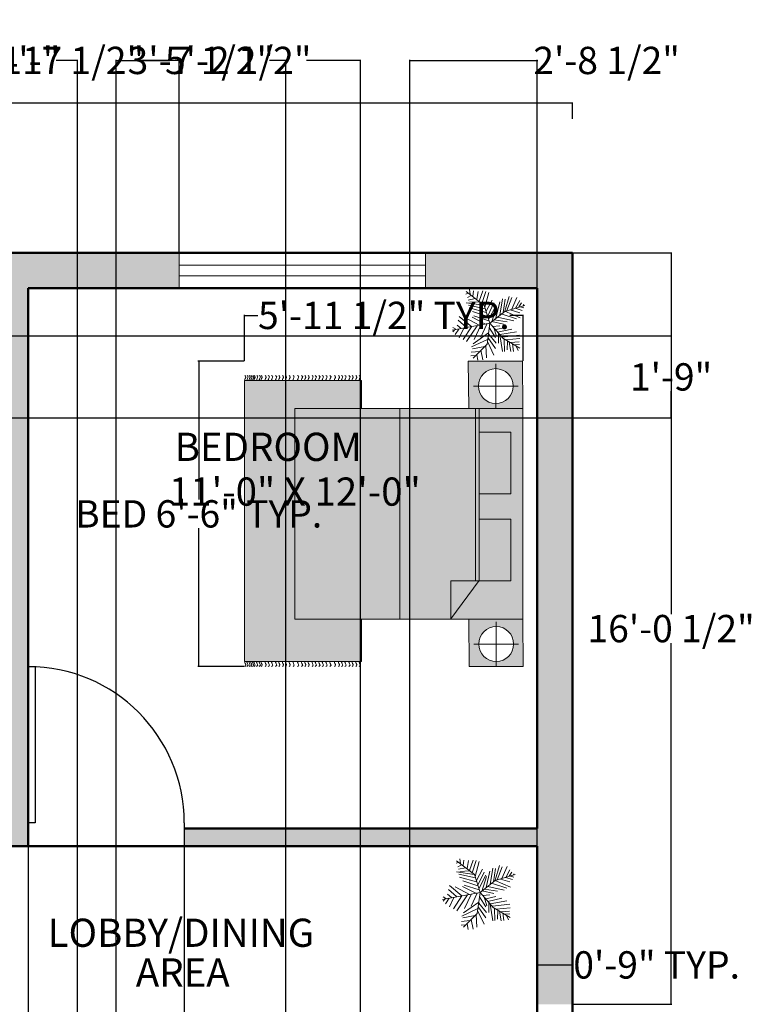
# Model space of a CAD drawing. Units: inches. Extents: x 2974 to 3443, y 2405 to 2963.
# Tile 13 of 13: x 3243 to 3430, y 2711 to 2963. Entities that reach past the tile are written whole.
import ezdxf

# ---------------------------------------------------------------- set-up
doc = ezdxf.new("R2010")
doc.units = ezdxf.units.IN
doc.header["$MEASUREMENT"] = 0
doc.layers.get('0').update_dxf_attribs({"color": 251})
for name, color, linetype, lineweight in [('A-ANNO-DIMS', 2, 'Continuous', 18), ('A-AREA-IDEN', 250, 'Continuous', 25), ('A-DOOR', 32, 'Continuous', 25), ('A-WALL-PATT', 252, 'Continuous', 13), ('furniture', 32, 'Continuous', 18), ('greenary', 106, 'Continuous', 13), ('walls', 250, 'Continuous', 50), ('windows', 159, 'Continuous', 20)]:
    doc.layers.add(name, color=color, linetype=linetype, lineweight=lineweight)
doc.layers.add('A-FURN-PATT', color=254, linetype='Continuous', lineweight=13, true_color=0xfeeab9)
doc.styles.get("Standard").update_dxf_attribs({"font": 'arial.ttf'})
doc.dimstyles.get("Standard").update_dxf_attribs({"dimtxt": 7, "dimasz": 0.18, "dimexe": 0.18, "dimexo": 0.0625, "dimgap": 0.09, "dimtad": 0, "dimtih": 1, "dimtoh": 1, "dimzin": 0, "dimdsep": 46, "dimlunit": 3, "dimtxsty": 'Standard', "dimcen": 0.09, "dimadec": 0, "dimazin": 0, "dimtfac": 1, "dimtofl": 0, "dimtmove": 0, "dimatfit": 3, "dimfxl": 1, "dimtolj": 1, "dimtzin": 0, "dimarcsym": 0})

# ---------------------------------------------------------------- blocks, each defined once
blk = doc.blocks.new('*U2')
for p, q in [((0, 0), (0, -6)), ((40, 0), (40, -6))]:
    blk.add_line(p, q)
blk.add_lwpolyline([(0, 0), (0, 40), (1.75, 40), (1.75, 0)], close=True)
blk.add_arc((0, 0), 40, 0, 90)
blk = doc.blocks.new('CARPET')
at = {"layer": 'furniture'}
for p, q in [((-51.53, -98.11), (-51.53, -55.12)), ((-51.53, -55.12), (-41.27, -55.12)), ((36, -55.12), (51.55, -55.12)), ((51.55, -55.12), (51.55, -98.11)), ((51.55, -98.11), (-51.53, -98.11))]:
    blk.add_line(p, q, dxfattribs=at)
for points, knots in [([(-53.37, -55.99), (-53.22, -55.8), (-52.9, -55.41), (-52.34, -55.8), (-51.89, -56.08), (-51.65, -55.91), (-51.53, -55.83)], [0, 0, 0, 0, 0.653278, 1.290138, 1.740457, 2.114451, 2.114451, 2.114451, 2.114451]), ([(-53.37, -57.26), (-53.22, -57.07), (-52.9, -56.67), (-52.34, -57.07), (-51.89, -57.35), (-51.65, -57.17), (-51.53, -57.1)], [0, 0, 0, 0, 0.653278, 1.290138, 1.740457, 2.114451, 2.114451, 2.114451, 2.114451]), ([(53.37, -55.99), (53.22, -55.8), (52.9, -55.41), (52.34, -55.8), (51.89, -56.08), (51.65, -55.91), (51.53, -55.83)], [0, 0, 0, 0, 0.653278, 1.290138, 1.740457, 2.114451, 2.114451, 2.114451, 2.114451]), ([(53.37, -57.26), (53.22, -57.07), (52.9, -56.67), (52.34, -57.07), (51.89, -57.35), (51.65, -57.17), (51.53, -57.1)], [0, 0, 0, 0, 0.653278, 1.290138, 1.740457, 2.114451, 2.114451, 2.114451, 2.114451]), ([(-53.37, -58.59), (-53.22, -58.4), (-52.9, -58.01), (-52.34, -58.4), (-51.89, -58.68), (-51.65, -58.5), (-51.53, -58.43)], [0, 0, 0, 0, 0.653278, 1.290138, 1.740457, 2.114451, 2.114451, 2.114451, 2.114451]), ([(-53.37, -59.78), (-53.22, -59.58), (-52.9, -59.19), (-52.34, -59.58), (-51.89, -59.86), (-51.65, -59.69), (-51.53, -59.61)], [0, 0, 0, 0, 0.653278, 1.290138, 1.740457, 2.114451, 2.114451, 2.114451, 2.114451]), ([(-53.37, -61.22), (-53.22, -61.02), (-52.9, -60.63), (-52.34, -61.02), (-51.89, -61.3), (-51.65, -61.13), (-51.53, -61.05)], [0, 0, 0, 0, 0.653278, 1.290138, 1.740457, 2.114451, 2.114451, 2.114451, 2.114451]), ([(53.37, -58.59), (53.22, -58.4), (52.9, -58.01), (52.34, -58.4), (51.89, -58.68), (51.65, -58.5), (51.53, -58.43)], [0, 0, 0, 0, 0.653278, 1.290138, 1.740457, 2.114451, 2.114451, 2.114451, 2.114451]), ([(53.37, -59.78), (53.22, -59.58), (52.9, -59.19), (52.34, -59.58), (51.89, -59.86), (51.65, -59.69), (51.53, -59.61)], [0, 0, 0, 0, 0.653278, 1.290138, 1.740457, 2.114451, 2.114451, 2.114451, 2.114451]), ([(53.37, -61.22), (53.22, -61.02), (52.9, -60.63), (52.34, -61.02), (51.89, -61.3), (51.65, -61.13), (51.53, -61.05)], [0, 0, 0, 0, 0.653278, 1.290138, 1.740457, 2.114451, 2.114451, 2.114451, 2.114451]), ([(-53.37, -62.44), (-53.22, -62.25), (-52.9, -61.86), (-52.34, -62.25), (-51.89, -62.53), (-51.65, -62.36), (-51.53, -62.28)], [0, 0, 0, 0, 0.653278, 1.290138, 1.740457, 2.114451, 2.114451, 2.114451, 2.114451]), ([(-53.37, -63.63), (-53.22, -63.43), (-52.9, -63.04), (-52.34, -63.43), (-51.89, -63.72), (-51.65, -63.54), (-51.53, -63.46)], [0, 0, 0, 0, 0.653278, 1.290138, 1.740457, 2.114451, 2.114451, 2.114451, 2.114451]), ([(-53.37, -65.07), (-53.22, -64.87), (-52.9, -64.48), (-52.34, -64.87), (-51.89, -65.15), (-51.65, -64.98), (-51.53, -64.9)], [0, 0, 0, 0, 0.653278, 1.290138, 1.740457, 2.114451, 2.114451, 2.114451, 2.114451]), ([(53.37, -62.44), (53.22, -62.25), (52.9, -61.86), (52.34, -62.25), (51.89, -62.53), (51.65, -62.36), (51.53, -62.28)], [0, 0, 0, 0, 0.653278, 1.290138, 1.740457, 2.114451, 2.114451, 2.114451, 2.114451]), ([(53.37, -63.63), (53.22, -63.43), (52.9, -63.04), (52.34, -63.43), (51.89, -63.72), (51.65, -63.54), (51.53, -63.46)], [0, 0, 0, 0, 0.653278, 1.290138, 1.740457, 2.114451, 2.114451, 2.114451, 2.114451]), ([(53.37, -65.07), (53.22, -64.87), (52.9, -64.48), (52.34, -64.87), (51.89, -65.15), (51.65, -64.98), (51.53, -64.9)], [0, 0, 0, 0, 0.653278, 1.290138, 1.740457, 2.114451, 2.114451, 2.114451, 2.114451]), ([(-53.37, -66.76), (-53.22, -66.56), (-52.9, -66.17), (-52.34, -66.56), (-51.89, -66.84), (-51.65, -66.67), (-51.53, -66.59)], [0, 0, 0, 0, 0.653278, 1.290138, 1.740457, 2.114451, 2.114451, 2.114451, 2.114451]), ([(-53.37, -68.2), (-53.22, -68), (-52.9, -67.61), (-52.34, -68), (-51.89, -68.28), (-51.65, -68.11), (-51.53, -68.03)], [0, 0, 0, 0, 0.653278, 1.290138, 1.740457, 2.114451, 2.114451, 2.114451, 2.114451]), ([(53.37, -66.76), (53.22, -66.56), (52.9, -66.17), (52.34, -66.56), (51.89, -66.84), (51.65, -66.67), (51.53, -66.59)], [0, 0, 0, 0, 0.653278, 1.290138, 1.740457, 2.114451, 2.114451, 2.114451, 2.114451]), ([(53.37, -68.2), (53.22, -68), (52.9, -67.61), (52.34, -68), (51.89, -68.28), (51.65, -68.11), (51.53, -68.03)], [0, 0, 0, 0, 0.653278, 1.290138, 1.740457, 2.114451, 2.114451, 2.114451, 2.114451]), ([(-53.37, -69.53), (-53.22, -69.33), (-52.9, -68.94), (-52.34, -69.33), (-51.89, -69.61), (-51.65, -69.44), (-51.53, -69.36)], [0, 0, 0, 0, 0.653278, 1.290138, 1.740457, 2.114451, 2.114451, 2.114451, 2.114451]), ([(-53.37, -70.79), (-53.22, -70.6), (-52.9, -70.21), (-52.34, -70.6), (-51.89, -70.88), (-51.65, -70.7), (-51.53, -70.63)], [0, 0, 0, 0, 0.653278, 1.290138, 1.740457, 2.114451, 2.114451, 2.114451, 2.114451]), ([(-53.37, -72.12), (-53.22, -71.93), (-52.9, -71.54), (-52.34, -71.93), (-51.89, -72.21), (-51.65, -72.04), (-51.53, -71.96)], [0, 0, 0, 0, 0.653278, 1.290138, 1.740457, 2.114451, 2.114451, 2.114451, 2.114451]), ([(53.37, -69.53), (53.22, -69.33), (52.9, -68.94), (52.34, -69.33), (51.89, -69.61), (51.65, -69.44), (51.53, -69.36)], [0, 0, 0, 0, 0.653278, 1.290138, 1.740457, 2.114451, 2.114451, 2.114451, 2.114451]), ([(53.37, -70.79), (53.22, -70.6), (52.9, -70.21), (52.34, -70.6), (51.89, -70.88), (51.65, -70.7), (51.53, -70.63)], [0, 0, 0, 0, 0.653278, 1.290138, 1.740457, 2.114451, 2.114451, 2.114451, 2.114451]), ([(53.37, -72.12), (53.22, -71.93), (52.9, -71.54), (52.34, -71.93), (51.89, -72.21), (51.65, -72.04), (51.53, -71.96)], [0, 0, 0, 0, 0.653278, 1.290138, 1.740457, 2.114451, 2.114451, 2.114451, 2.114451]), ([(-53.37, -73.31), (-53.22, -73.11), (-52.9, -72.72), (-52.34, -73.11), (-51.89, -73.4), (-51.65, -73.22), (-51.53, -73.14)], [0, 0, 0, 0, 0.653278, 1.290138, 1.740457, 2.114451, 2.114451, 2.114451, 2.114451]), ([(-53.37, -74.75), (-53.22, -74.55), (-52.9, -74.16), (-52.34, -74.55), (-51.89, -74.83), (-51.65, -74.66), (-51.53, -74.58)], [0, 0, 0, 0, 0.653278, 1.290138, 1.740457, 2.114451, 2.114451, 2.114451, 2.114451]), ([(-53.37, -75.98), (-53.22, -75.78), (-52.9, -75.39), (-52.34, -75.78), (-51.89, -76.06), (-51.65, -75.89), (-51.53, -75.81)], [0, 0, 0, 0, 0.653278, 1.290138, 1.740457, 2.114451, 2.114451, 2.114451, 2.114451]), ([(53.37, -73.31), (53.22, -73.11), (52.9, -72.72), (52.34, -73.11), (51.89, -73.4), (51.65, -73.22), (51.53, -73.14)], [0, 0, 0, 0, 0.653278, 1.290138, 1.740457, 2.114451, 2.114451, 2.114451, 2.114451]), ([(53.37, -74.75), (53.22, -74.55), (52.9, -74.16), (52.34, -74.55), (51.89, -74.83), (51.65, -74.66), (51.53, -74.58)], [0, 0, 0, 0, 0.653278, 1.290138, 1.740457, 2.114451, 2.114451, 2.114451, 2.114451]), ([(53.37, -75.98), (53.22, -75.78), (52.9, -75.39), (52.34, -75.78), (51.89, -76.06), (51.65, -75.89), (51.53, -75.81)], [0, 0, 0, 0, 0.653278, 1.290138, 1.740457, 2.114451, 2.114451, 2.114451, 2.114451]), ([(-53.37, -77.16), (-53.22, -76.96), (-52.9, -76.57), (-52.34, -76.96), (-51.89, -77.25), (-51.65, -77.07), (-51.53, -76.99)], [0, 0, 0, 0, 0.653278, 1.290138, 1.740457, 2.114451, 2.114451, 2.114451, 2.114451]), ([(-53.37, -78.6), (-53.22, -78.4), (-52.9, -78.01), (-52.34, -78.4), (-51.89, -78.68), (-51.65, -78.51), (-51.53, -78.43)], [0, 0, 0, 0, 0.653278, 1.290138, 1.740457, 2.114451, 2.114451, 2.114451, 2.114451]), ([(53.37, -77.16), (53.22, -76.96), (52.9, -76.57), (52.34, -76.96), (51.89, -77.25), (51.65, -77.07), (51.53, -76.99)], [0, 0, 0, 0, 0.653278, 1.290138, 1.740457, 2.114451, 2.114451, 2.114451, 2.114451]), ([(53.37, -78.6), (53.22, -78.4), (52.9, -78.01), (52.34, -78.4), (51.89, -78.68), (51.65, -78.51), (51.53, -78.43)], [0, 0, 0, 0, 0.653278, 1.290138, 1.740457, 2.114451, 2.114451, 2.114451, 2.114451]), ([(-53.37, -80.29), (-53.22, -80.09), (-52.9, -79.7), (-52.34, -80.09), (-51.89, -80.37), (-51.65, -80.2), (-51.53, -80.12)], [0, 0, 0, 0, 0.653278, 1.290138, 1.740457, 2.114451, 2.114451, 2.114451, 2.114451]), ([(-53.37, -81.73), (-53.22, -81.53), (-52.9, -81.14), (-52.34, -81.53), (-51.89, -81.81), (-51.65, -81.64), (-51.53, -81.56)], [0, 0, 0, 0, 0.653278, 1.290138, 1.740457, 2.114451, 2.114451, 2.114451, 2.114451]), ([(-53.37, -83.06), (-53.22, -82.86), (-52.9, -82.47), (-52.34, -82.86), (-51.89, -83.14), (-51.65, -82.97), (-51.53, -82.89)], [0, 0, 0, 0, 0.653278, 1.290138, 1.740457, 2.114451, 2.114451, 2.114451, 2.114451]), ([(53.37, -80.29), (53.22, -80.09), (52.9, -79.7), (52.34, -80.09), (51.89, -80.37), (51.65, -80.2), (51.53, -80.12)], [0, 0, 0, 0, 0.653278, 1.290138, 1.740457, 2.114451, 2.114451, 2.114451, 2.114451]), ([(53.37, -81.73), (53.22, -81.53), (52.9, -81.14), (52.34, -81.53), (51.89, -81.81), (51.65, -81.64), (51.53, -81.56)], [0, 0, 0, 0, 0.653278, 1.290138, 1.740457, 2.114451, 2.114451, 2.114451, 2.114451]), ([(53.37, -83.06), (53.22, -82.86), (52.9, -82.47), (52.34, -82.86), (51.89, -83.14), (51.65, -82.97), (51.53, -82.89)], [0, 0, 0, 0, 0.653278, 1.290138, 1.740457, 2.114451, 2.114451, 2.114451, 2.114451]), ([(-53.37, -84.18), (-53.22, -83.99), (-52.9, -83.6), (-52.34, -83.99), (-51.89, -84.27), (-51.65, -84.09), (-51.53, -84.02)], [0, 0, 0, 0, 0.653278, 1.290138, 1.740457, 2.114451, 2.114451, 2.114451, 2.114451]), ([(-53.37, -85.51), (-53.22, -85.32), (-52.9, -84.93), (-52.34, -85.32), (-51.89, -85.6), (-51.65, -85.42), (-51.53, -85.35)], [0, 0, 0, 0, 0.653278, 1.290138, 1.740457, 2.114451, 2.114451, 2.114451, 2.114451]), ([(-53.37, -86.7), (-53.22, -86.5), (-52.9, -86.11), (-52.34, -86.5), (-51.89, -86.78), (-51.65, -86.61), (-51.53, -86.53)], [0, 0, 0, 0, 0.653278, 1.290138, 1.740457, 2.114451, 2.114451, 2.114451, 2.114451]), ([(53.37, -84.18), (53.22, -83.99), (52.9, -83.6), (52.34, -83.99), (51.89, -84.27), (51.65, -84.09), (51.53, -84.02)], [0, 0, 0, 0, 0.653278, 1.290138, 1.740457, 2.114451, 2.114451, 2.114451, 2.114451]), ([(53.37, -85.51), (53.22, -85.32), (52.9, -84.93), (52.34, -85.32), (51.89, -85.6), (51.65, -85.42), (51.53, -85.35)], [0, 0, 0, 0, 0.653278, 1.290138, 1.740457, 2.114451, 2.114451, 2.114451, 2.114451]), ([(53.37, -86.7), (53.22, -86.5), (52.9, -86.11), (52.34, -86.5), (51.89, -86.78), (51.65, -86.61), (51.53, -86.53)], [0, 0, 0, 0, 0.653278, 1.290138, 1.740457, 2.114451, 2.114451, 2.114451, 2.114451]), ([(-53.37, -88.14), (-53.22, -87.94), (-52.9, -87.55), (-52.34, -87.94), (-51.89, -88.22), (-51.65, -88.05), (-51.53, -87.97)], [0, 0, 0, 0, 0.653278, 1.290138, 1.740457, 2.114451, 2.114451, 2.114451, 2.114451]), ([(-53.37, -89.36), (-53.22, -89.17), (-52.9, -88.78), (-52.34, -89.17), (-51.89, -89.45), (-51.65, -89.28), (-51.53, -89.2)], [0, 0, 0, 0, 0.653278, 1.290138, 1.740457, 2.114451, 2.114451, 2.114451, 2.114451]), ([(-53.37, -90.55), (-53.22, -90.35), (-52.9, -89.96), (-52.34, -90.35), (-51.89, -90.64), (-51.65, -90.46), (-51.53, -90.38)], [0, 0, 0, 0, 0.653278, 1.290138, 1.740457, 2.114451, 2.114451, 2.114451, 2.114451]), ([(53.37, -88.14), (53.22, -87.94), (52.9, -87.55), (52.34, -87.94), (51.89, -88.22), (51.65, -88.05), (51.53, -87.97)], [0, 0, 0, 0, 0.653278, 1.290138, 1.740457, 2.114451, 2.114451, 2.114451, 2.114451]), ([(53.37, -89.36), (53.22, -89.17), (52.9, -88.78), (52.34, -89.17), (51.89, -89.45), (51.65, -89.28), (51.53, -89.2)], [0, 0, 0, 0, 0.653278, 1.290138, 1.740457, 2.114451, 2.114451, 2.114451, 2.114451]), ([(53.37, -90.55), (53.22, -90.35), (52.9, -89.96), (52.34, -90.35), (51.9, -90.63), (51.66, -90.47), (51.55, -90.4)], [0, 0, 0, 0, 0.653278, 1.290138, 1.740457, 2.0926, 2.0926, 2.0926, 2.0926]), ([(-53.37, -91.99), (-53.22, -91.79), (-52.9, -91.4), (-52.34, -91.79), (-51.89, -92.07), (-51.65, -91.9), (-51.53, -91.82)], [0, 0, 0, 0, 0.653278, 1.290138, 1.740457, 2.114451, 2.114451, 2.114451, 2.114451]), ([(-53.37, -92.69), (-53.22, -92.48), (-52.9, -92.08), (-52.35, -92.49), (-51.89, -92.77), (-51.65, -92.6), (-51.53, -92.52)], [0, 0, 0, 0, 0.663904, 1.307406, 1.757725, 2.131719, 2.131719, 2.131719, 2.131719]), ([(-53.37, -93.61), (-53.22, -93.42), (-52.9, -93.03), (-52.34, -93.42), (-51.89, -93.7), (-51.65, -93.52), (-51.53, -93.45)], [0, 0, 0, 0, 0.653278, 1.290138, 1.740457, 2.114451, 2.114451, 2.114451, 2.114451]), ([(53.37, -91.99), (53.22, -91.79), (52.9, -91.4), (52.34, -91.79), (51.9, -92.07), (51.66, -91.91), (51.55, -91.83)], [0, 0, 0, 0, 0.653278, 1.290138, 1.740457, 2.0926, 2.0926, 2.0926, 2.0926]), ([(53.37, -92.69), (53.22, -92.49), (52.9, -92.09), (52.34, -92.49), (51.9, -92.77), (51.66, -92.61), (51.55, -92.53)], [0, 0, 0, 0, 0.656792, 1.295826, 1.746145, 2.098292, 2.098292, 2.098292, 2.098292]), ([(53.37, -93.66), (53.22, -93.46), (52.9, -93.07), (52.34, -93.46), (51.9, -93.74), (51.66, -93.58), (51.55, -93.5)], [0, 0, 0, 0, 0.653278, 1.290138, 1.740457, 2.0926, 2.0926, 2.0926, 2.0926]), ([(-53.37, -94.55), (-53.22, -94.35), (-52.9, -93.96), (-52.34, -94.35), (-51.89, -94.63), (-51.65, -94.46), (-51.53, -94.38)], [0, 0, 0, 0, 0.653278, 1.290138, 1.740457, 2.114451, 2.114451, 2.114451, 2.114451]), ([(-53.37, -95.05), (-53.22, -94.85), (-52.9, -94.46), (-52.34, -94.85), (-51.89, -95.14), (-51.65, -94.96), (-51.53, -94.88)], [0, 0, 0, 0, 0.653278, 1.290138, 1.740457, 2.114451, 2.114451, 2.114451, 2.114451]), ([(-53.37, -95.73), (-53.22, -95.54), (-52.9, -95.15), (-52.34, -95.54), (-51.89, -95.82), (-51.65, -95.65), (-51.53, -95.57)], [0, 0, 0, 0, 0.653278, 1.290138, 1.740457, 2.114451, 2.114451, 2.114451, 2.114451]), ([(-53.37, -96.38), (-53.22, -96.18), (-52.9, -95.79), (-52.34, -96.18), (-51.89, -96.47), (-51.65, -96.29), (-51.53, -96.21)], [0, 0, 0, 0, 0.653278, 1.290138, 1.740457, 2.114451, 2.114451, 2.114451, 2.114451]), ([(-53.37, -97.17), (-53.22, -96.98), (-52.9, -96.59), (-52.34, -96.98), (-51.89, -97.26), (-51.65, -97.08), (-51.53, -97.01)], [0, 0, 0, 0, 0.653278, 1.290138, 1.740457, 2.114451, 2.114451, 2.114451, 2.114451]), ([(53.37, -95.78), (53.22, -95.58), (52.9, -95.19), (52.34, -95.58), (51.89, -95.86), (51.65, -95.69), (51.53, -95.61)], [0, 0, 0, 0, 0.653278, 1.290138, 1.740457, 2.114451, 2.114451, 2.114451, 2.114451]), ([(53.37, -96.43), (53.22, -96.23), (52.9, -95.84), (52.34, -96.23), (51.89, -96.51), (51.65, -96.34), (51.53, -96.26)], [0, 0, 0, 0, 0.653278, 1.290138, 1.740457, 2.114451, 2.114451, 2.114451, 2.114451]), ([(53.37, -97.22), (53.22, -97.02), (52.9, -96.63), (52.34, -97.02), (51.89, -97.3), (51.65, -97.13), (51.53, -97.05)], [0, 0, 0, 0, 0.653278, 1.290138, 1.740457, 2.114451, 2.114451, 2.114451, 2.114451]), ([(53.37, -94.59), (53.22, -94.4), (52.9, -94.01), (52.34, -94.4), (51.9, -94.68), (51.66, -94.51), (51.55, -94.44)], [0, 0, 0, 0, 0.653278, 1.290138, 1.740457, 2.0926, 2.0926, 2.0926, 2.0926]), ([(53.37, -95.1), (53.22, -94.9), (52.9, -94.51), (52.34, -94.9), (51.9, -95.18), (51.66, -95.02), (51.55, -94.94)], [0, 0, 0, 0, 0.653278, 1.290138, 1.740457, 2.0926, 2.0926, 2.0926, 2.0926]), ([(-53.37, -97.99), (-53.22, -97.79), (-52.9, -97.4), (-52.34, -97.79), (-51.89, -98.08), (-51.65, -97.9), (-51.53, -97.82)], [0, 0, 0, 0, 0.653278, 1.290138, 1.740457, 2.114451, 2.114451, 2.114451, 2.114451]), ([(53.37, -97.99), (53.22, -97.79), (52.9, -97.4), (52.34, -97.79), (51.89, -98.08), (51.65, -97.9), (51.53, -97.82)], [0, 0, 0, 0, 0.653278, 1.290138, 1.740457, 2.114451, 2.114451, 2.114451, 2.114451])]:
    blk.add_open_spline(points, degree=3, knots=knots, dxfattribs=at)
blk = doc.blocks.new('A$C58D270C6')
at = {"layer": 'furniture'}
for p, q in [((9.09, 124.13), (9.09, 108.87)), ((1.46, 116.5), (16.73, 116.5)), ((14.97, 94.84), (24.62, 107.92)), ((24.62, 94.93), (24.62, 107.92)), ((42.08, 108), (42.08, 36)), ((14.97, 94.93), (24.62, 94.93)), ((14.97, 94.84), (14.97, 36)), ((16.22, 94.93), (16.22, 36)), ((9.25, 36), (9.25, 20.74)), ((1.62, 28.37), (16.88, 28.37))]:
    blk.add_line(p, q, dxfattribs=at)
for points in [[(18.5, 108), (18.34, 124.13), (-0.16, 124.13), (0, 108)], [(0, 108), (77.91, 108), (77.91, 36), (0, 36)], [(4.09, 94.93), (14.97, 94.93), (14.97, 73.83), (4.09, 73.83)], [(4.09, 65.23), (14.97, 65.23), (14.97, 44.13), (4.09, 44.13)], [(18.65, 19.87), (18.5, 36), (0, 36), (0.16, 19.87)]]:
    blk.add_lwpolyline(points, close=True, dxfattribs=at)
for centre in [(9.09, 116.5), (9.25, 28.37)]:
    blk.add_circle(centre, 5.95, dxfattribs=at)
at = {"layer": 'furniture', "xscale": 0.9312884925094044, "yscale": 0.9312884925094044, "zscale": 0.9312884925094044, "rotation": 90}
blk.add_blockref('CARPET', (3.79, 74.47), dxfattribs=at)
blk = doc.blocks.new('*U13')
for p, q in [((-7.288, 39.707), (-21.778, 46.673)), ((-8.737, 47.138), (-17.069, 52.711)), ((-10.186, 53.64), (-13.084, 55.962)), ((0, 0), (-10.5, 57)), ((-9.099, 51.782), (-6.563, 55.962)), ((-7.65, 43.423), (-2.578, 49.46)), ((-5.839, 35.992), (4.667, 48.067)), ((-5.114, 27.632), (10.463, 46.673)), ((-3.665, 19.273), (-27.574, 35.527)), ((-5.114, 28.097), (-24.676, 40.636)), ((-2.941, 16.486), (8.652, 37.85)), ((16.259, 5.805), (23.142, 31.348)), ((22.055, 7.198), (27.489, 32.277)), ((27, 9), (48, 36)), ((27.127, 9.056), (31.112, 35.992)), ((31.836, 30.883), (32.561, 16.486)), ((35.096, 32.741), (37.27, 22.524)), ((38.719, 34.134), (41.979, 28.561)), ((43.791, 29.954), (51.036, 30.883)), ((44.153, 36.456), (45.239, 32.741)), ((-47.498, 19.737), (-55.83, 18.344)), ((-31.5, 4.5), (-52.5, 25.5)), ((-48.585, 21.131), (-49.309, 29.026)), ((-43.513, 28.561), (-42.427, 15.558)), ((-38.442, 26.239), (-34.819, 7.663)), ((-35.544, 28.097), (-24.314, 3.947)), ((-14.533, 2.09), (-30.834, 25.31)), ((-24.314, 23.917), (-2.941, 13.7)), ((-1.129, 6.734), (9.014, 26.704)), ((3.942, 1.625), (11.187, 24.381)), ((10.101, 3.483), (17.708, 26.239)), ((33.285, 16.486), (48.862, 10.913)), ((36.183, 19.737), (48.137, 17.88)), ((40.53, 25.775), (48.862, 24.846)), ((-40.615, 13.7), (-55.105, 10.913)), ((-33.37, 6.269), (-52.207, 5.34)), ((-28.299, 3.483), (-47.86, -5.805)), ((-21.416, 3.018), (-38.079, -8.128)), ((0, 0), (-31.5, 4.5)), ((-15.982, 2.09), (-30.11, -9.521)), ((0, 0), (-22.5, -19.5)), ((-6.563, 1.161), (-21.416, -8.128)), ((-20.691, 13.7), (-1.129, 4.876)), ((0, 0), (27, 9)), ((0, 0), (18, -22.5)), ((6.478, 1.625), (26.04, -8.592)), ((11.187, 3.483), (30.749, -5.805)), ((18.07, 5.805), (35.096, -3.483)), ((24.229, 7.663), (46.688, 1.625)), ((29.662, 12.307), (48.137, 6.269)), ((-15.257, -12.772), (-30.11, -12.772)), ((-6.563, -5.805), (-19.967, -9.985)), ((-13.446, -11.378), (-8.737, -32.741)), ((-9.461, -8.592), (-6.201, -23.453)), ((-4.752, -3.483), (-3.665, -14.629)), ((2.493, -3.019), (-1.491, -20.202)), ((1.769, -2.555), (24.229, -9.521)), ((5.029, -6.27), (2.131, -25.775)), ((9.014, -11.378), (3.58, -35.992)), ((7.565, -9.056), (32.198, -14.629)), ((-17.431, -15.094), (-42.789, -18.809)), ((-28.299, -29.026), (-42.789, -31.348)), ((-24.314, -21.596), (-42.427, -22.06)), ((-26.849, -26.24), (-40.253, -25.775)), ((-22.5, -19.5), (-37.5, -45)), ((-25.038, -23.918), (-22.865, -45.281)), ((-20.691, -18.345), (-17.793, -44.352)), ((-17.069, -15.094), (-12.721, -40.172)), ((14.085, -16.951), (6.478, -40.172)), ((18.07, -22.524), (8.289, -45.745)), ((12.274, -15.094), (36.907, -18.809)), ((16.259, -19.738), (36.183, -22.989)), ((18, -22.5), (27, -52.5)), ((18.433, -22.524), (40.53, -29.026)), ((19.157, -25.311), (38.719, -33.206)), ((-30.834, -34.135), (-42.427, -35.528)), ((-34.457, -39.708), (-40.978, -42.494)), ((-32.646, -36.921), (-31.921, -44.352)), ((-29.023, -30.884), (-27.936, -43.887)), ((20.244, -30.419), (15.897, -44.816)), ((22.78, -37.85), (19.519, -48.532)), ((21.331, -32.741), (39.081, -40.636)), ((22.78, -38.314), (34.372, -44.816)), ((24.591, -43.423), (30.749, -47.603)), ((24.591, -45.745), (23.142, -50.854)), ((26.764, -49.925), (28.213, -50.854))]:
    blk.add_line(p, q)
blk = doc.blocks.new('*D19')
at = {"layer": 'A-ANNO-DIMS', "color": 0, "lineweight": -2, "transparency": 16777216}
for p, q in [((3042.33, 2937.52), (3042.33, 2941.76)), ((3384.33, 2937.52), (3384.33, 2941.76)), ((3042.51, 2941.58), (3194.36, 2941.58)), ((3384.15, 2941.58), (3232.3, 2941.58))]:
    blk.add_line(p, q, dxfattribs=at)
at = {"layer": 'A-ANNO-DIMS', "color": 0, "transparency": 16777216}
for points in [[(3042.51, 2941.61), (3042.51, 2941.55), (3042.33, 2941.58)], [(3384.15, 2941.61), (3384.15, 2941.55), (3384.33, 2941.58)]]:
    blk.add_solid(points, dxfattribs=at)
at = {"layer": 'Defpoints', "color": 0, "transparency": 16777216}
for p in [(3384.33, 2941.58), (3042.33, 2937.45), (3384.33, 2937.45)]:
    blk.add_point(p, dxfattribs=at)
at = {"layer": 'A-ANNO-DIMS', "color": 0, "transparency": 16777216, "insert": (3213.33, 2941.58), "char_height": 7, "attachment_point": 5}
blk.add_mtext('\\A1;28\'-6.00"', dxfattribs=at)
blk = doc.blocks.new('WIN-63IN')
for p, q in [((0, 0), (0, -9)), ((63.13, 0), (0, 0)), ((0, 0), (0, -3.12)), ((63.13, -9), (63.13, 0)), ((0, -3.12), (63.13, -3.12)), ((63.13, -3.12), (63.13, -5.89)), ((63.13, -5.89), (0, -5.89)), ((0, -9), (63.13, -9))]:
    blk.add_line(p, q)
blk = doc.blocks.new('*D32')
at = {"layer": 'A-ANNO-DIMS', "color": 0, "lineweight": -2, "transparency": 16777216}
for p, q in [((3375.33, 2710.72), (3375.33, 2720.93)), ((3375.51, 2720.75), (3384.15, 2720.75)), ((3384.33, 2710.72), (3384.33, 2720.93)), ((3384.33, 2720.75), (3384.51, 2720.75))]:
    blk.add_line(p, q, dxfattribs=at)
at = {"layer": 'A-ANNO-DIMS', "color": 0, "transparency": 16777216}
for points in [[(3375.51, 2720.78), (3375.51, 2720.72), (3375.33, 2720.75)], [(3384.15, 2720.78), (3384.15, 2720.72), (3384.33, 2720.75)]]:
    blk.add_solid(points, dxfattribs=at)
at = {"layer": 'Defpoints', "color": 0, "transparency": 16777216}
for p in [(3384.33, 2720.75), (3375.33, 2710.65), (3384.33, 2710.65)]:
    blk.add_point(p, dxfattribs=at)
at = {"layer": 'A-ANNO-DIMS', "color": 0, "transparency": 16777216, "insert": (3405.93, 2720.75), "char_height": 7, "attachment_point": 5}
blk.add_mtext('\\A1;0\'-9" TYP.', dxfattribs=at)
blk = doc.blocks.new('*D33')
at = {"layer": 'A-ANNO-DIMS', "color": 0, "lineweight": -2, "transparency": 16777216}
for p, q in [((3300.2, 2875.44), (3288.35, 2875.44)), ((3288.53, 2875.26), (3288.53, 2839.99)), ((3288.53, 2797.38), (3288.53, 2832.66)), ((3300.2, 2797.2), (3288.35, 2797.2))]:
    blk.add_line(p, q, dxfattribs=at)
at = {"layer": 'A-ANNO-DIMS', "color": 0, "transparency": 16777216}
for points in [[(3288.5, 2875.26), (3288.56, 2875.26), (3288.53, 2875.44)], [(3288.5, 2797.38), (3288.56, 2797.38), (3288.53, 2797.2)]]:
    blk.add_solid(points, dxfattribs=at)
at = {"layer": 'Defpoints', "color": 0, "transparency": 16777216}
for p in [(3300.26, 2875.44), (3288.53, 2797.2), (3300.26, 2797.2)]:
    blk.add_point(p, dxfattribs=at)
at = {"layer": 'A-ANNO-DIMS', "color": 0, "transparency": 16777216, "insert": (3288.53, 2836.32), "char_height": 7, "attachment_point": 5}
blk.add_mtext('\\A1;BED 6\'-6" TYP.', dxfattribs=at)
blk = doc.blocks.new('*D34')
at = {"layer": 'A-ANNO-DIMS', "color": 0, "lineweight": -2, "transparency": 16777216}
for p, q in [((3300.26, 2875.5), (3300.26, 2887.35)), ((3300.44, 2887.17), (3303.7, 2887.17)), ((3371.57, 2887.17), (3368.3, 2887.17)), ((3371.75, 2875.5), (3371.75, 2887.35))]:
    blk.add_line(p, q, dxfattribs=at)
at = {"layer": 'A-ANNO-DIMS', "color": 0, "transparency": 16777216}
for points in [[(3300.44, 2887.2), (3300.44, 2887.14), (3300.26, 2887.17)], [(3371.57, 2887.2), (3371.57, 2887.14), (3371.75, 2887.17)]]:
    blk.add_solid(points, dxfattribs=at)
at = {"layer": 'Defpoints', "color": 0, "transparency": 16777216}
for p in [(3300.26, 2887.17), (3300.26, 2875.44), (3371.75, 2875.44)]:
    blk.add_point(p, dxfattribs=at)
at = {"layer": 'A-ANNO-DIMS', "color": 0, "transparency": 16777216, "insert": (3336, 2887.17), "char_height": 7, "attachment_point": 5}
blk.add_mtext('\\A1;5\'-11 1/2" TYP.', dxfattribs=at)
blk = doc.blocks.new('*D53')
at = {"layer": 'A-ANNO-DIMS', "color": 0, "lineweight": -2, "transparency": 16777216}
for p, q in [((3227.95, 2903.25), (3227.95, 2952.68)), ((3228.13, 2952.5), (3238.07, 2952.5)), ((3283.38, 2952.5), (3273.45, 2952.5)), ((3283.56, 2903.25), (3283.56, 2952.68))]:
    blk.add_line(p, q, dxfattribs=at)
at = {"layer": 'A-ANNO-DIMS', "color": 0, "transparency": 16777216}
for points in [[(3228.13, 2952.53), (3228.13, 2952.47), (3227.95, 2952.5)], [(3283.38, 2952.53), (3283.38, 2952.47), (3283.56, 2952.5)]]:
    blk.add_solid(points, dxfattribs=at)
at = {"layer": 'Defpoints', "color": 0, "transparency": 16777216}
for p in [(3283.56, 2952.5), (3227.95, 2903.19), (3283.56, 2903.19)]:
    blk.add_point(p, dxfattribs=at)
at = {"layer": 'A-ANNO-DIMS', "color": 0, "transparency": 16777216, "insert": (3255.76, 2952.5), "char_height": 7, "attachment_point": 5}
blk.add_mtext('\\A1;4\'-7 1/2"', dxfattribs=at)
blk = doc.blocks.new('*D56')
at = {"layer": 'A-ANNO-DIMS', "color": 0, "lineweight": -2, "transparency": 16777216}
for p, q in [((3384.39, 2903.19), (3409.82, 2903.19)), ((3409.64, 2903.01), (3409.64, 2810.63)), ((3409.64, 2710.83), (3409.64, 2803.21)), ((3384.39, 2710.65), (3409.82, 2710.65))]:
    blk.add_line(p, q, dxfattribs=at)
at = {"layer": 'A-ANNO-DIMS', "color": 0, "transparency": 16777216}
for points in [[(3409.61, 2903.01), (3409.67, 2903.01), (3409.64, 2903.19)], [(3409.61, 2710.83), (3409.67, 2710.83), (3409.64, 2710.65)]]:
    blk.add_solid(points, dxfattribs=at)
at = {"layer": 'Defpoints', "color": 0, "transparency": 16777216}
for p in [(3384.33, 2903.19), (3384.33, 2710.65), (3409.64, 2710.65)]:
    blk.add_point(p, dxfattribs=at)
at = {"layer": 'A-ANNO-DIMS', "color": 0, "transparency": 16777216, "insert": (3409.64, 2806.92), "char_height": 7, "attachment_point": 5}
blk.add_mtext('\\A1;16\'-0 1/2"', dxfattribs=at)
blk = doc.blocks.new('*D61')
at = {"layer": 'A-ANNO-DIMS', "color": 0, "lineweight": -2, "transparency": 16777216}
for p, q in [((3222.29, 2555.25), (3222.29, 2952.68)), ((3222.47, 2952.5), (3227.69, 2952.5)), ((3257.25, 2952.5), (3252.03, 2952.5)), ((3257.43, 2555.25), (3257.43, 2952.68))]:
    blk.add_line(p, q, dxfattribs=at)
at = {"layer": 'A-ANNO-DIMS', "color": 0, "transparency": 16777216}
for points in [[(3222.47, 2952.53), (3222.47, 2952.47), (3222.29, 2952.5)], [(3257.25, 2952.53), (3257.25, 2952.47), (3257.43, 2952.5)]]:
    blk.add_solid(points, dxfattribs=at)
at = {"layer": 'Defpoints', "color": 0, "transparency": 16777216}
for p in [(3257.43, 2952.5), (3222.29, 2555.19), (3257.43, 2555.19)]:
    blk.add_point(p, dxfattribs=at)
at = {"layer": 'A-ANNO-DIMS', "color": 0, "transparency": 16777216, "insert": (3239.86, 2952.5), "char_height": 7, "attachment_point": 5}
blk.add_mtext('\\A1;2\'-11"', dxfattribs=at)
blk = doc.blocks.new('*D62')
at = {"layer": 'A-ANNO-DIMS', "color": 0, "lineweight": -2, "transparency": 16777216}
for p, q in [((3267.33, 2609.25), (3267.33, 2952.68)), ((3267.51, 2952.5), (3281.12, 2952.5)), ((3329.82, 2952.5), (3316.21, 2952.5)), ((3330, 2609.25), (3330, 2952.68))]:
    blk.add_line(p, q, dxfattribs=at)
at = {"layer": 'A-ANNO-DIMS', "color": 0, "transparency": 16777216}
for points in [[(3267.51, 2952.53), (3267.51, 2952.47), (3267.33, 2952.5)], [(3329.82, 2952.53), (3329.82, 2952.47), (3330, 2952.5)]]:
    blk.add_solid(points, dxfattribs=at)
at = {"layer": 'Defpoints', "color": 0, "transparency": 16777216}
for p in [(3330, 2952.5), (3267.33, 2609.19), (3330, 2609.19)]:
    blk.add_point(p, dxfattribs=at)
at = {"layer": 'A-ANNO-DIMS', "color": 0, "transparency": 16777216, "insert": (3298.66, 2952.5), "char_height": 7, "attachment_point": 5}
blk.add_mtext('\\A1;5\'-2 1/2"', dxfattribs=at)
blk = doc.blocks.new('*D63')
at = {"layer": 'A-ANNO-DIMS', "color": 0, "lineweight": -2, "transparency": 16777216}
for p, q in [((3244.83, 2751.13), (3244.83, 2414.92)), ((3284.83, 2751.13), (3284.83, 2414.92)), ((3245.01, 2415.1), (3255.43, 2415.1)), ((3284.65, 2415.1), (3274.22, 2415.1))]:
    blk.add_line(p, q, dxfattribs=at)
at = {"layer": 'A-ANNO-DIMS', "color": 0, "transparency": 16777216}
for points in [[(3245.01, 2415.13), (3245.01, 2415.07), (3244.83, 2415.1)], [(3284.65, 2415.13), (3284.65, 2415.07), (3284.83, 2415.1)]]:
    blk.add_solid(points, dxfattribs=at)
at = {"layer": 'Defpoints', "color": 0, "transparency": 16777216}
for p in [(3244.83, 2751.19), (3284.83, 2751.19), (3284.83, 2415.1)]:
    blk.add_point(p, dxfattribs=at)
at = {"layer": 'A-ANNO-DIMS', "color": 0, "transparency": 16777216, "insert": (3264.83, 2415.1), "char_height": 7, "attachment_point": 5}
blk.add_mtext('\\A1;3\'-4"', dxfattribs=at)
blk = doc.blocks.new('*D65')
at = {"layer": 'A-ANNO-DIMS', "color": 0, "lineweight": -2, "transparency": 16777216}
for p, q in [((3215.45, 2808.13), (3215.45, 2414.92)), ((3236.95, 2808.13), (3236.95, 2414.92)), ((3215.63, 2415.1), (3236.77, 2415.1)), ((3236.95, 2415.1), (3237.13, 2415.1))]:
    blk.add_line(p, q, dxfattribs=at)
at = {"layer": 'A-ANNO-DIMS', "color": 0, "transparency": 16777216}
for points in [[(3215.63, 2415.13), (3215.63, 2415.07), (3215.45, 2415.1)], [(3236.77, 2415.13), (3236.77, 2415.07), (3236.95, 2415.1)]]:
    blk.add_solid(points, dxfattribs=at)
at = {"layer": 'Defpoints', "color": 0, "transparency": 16777216}
for p in [(3215.45, 2808.19), (3236.95, 2808.19), (3236.95, 2415.1)]:
    blk.add_point(p, dxfattribs=at)
at = {"layer": 'A-ANNO-DIMS', "color": 0, "transparency": 16777216, "insert": (3254.35, 2415.1), "char_height": 7, "attachment_point": 5}
blk.add_mtext('\\A1;1\'-9 1/2"', dxfattribs=at)
blk = doc.blocks.new('*D70')
at = {"layer": 'A-ANNO-DIMS', "color": 0, "lineweight": -2, "transparency": 16777216}
for p, q in [((3075.39, 2881.91), (3409.82, 2881.91)), ((3409.64, 2881.73), (3409.64, 2875.08)), ((3409.64, 2861.09), (3409.64, 2867.75)), ((3075.39, 2860.91), (3409.82, 2860.91))]:
    blk.add_line(p, q, dxfattribs=at)
at = {"layer": 'A-ANNO-DIMS', "color": 0, "transparency": 16777216}
for points in [[(3409.61, 2881.73), (3409.67, 2881.73), (3409.64, 2881.91)], [(3409.61, 2861.09), (3409.67, 2861.09), (3409.64, 2860.91)]]:
    blk.add_solid(points, dxfattribs=at)
at = {"layer": 'Defpoints', "color": 0, "transparency": 16777216}
for p in [(3075.33, 2881.91), (3409.64, 2881.91), (3075.33, 2860.91)]:
    blk.add_point(p, dxfattribs=at)
at = {"layer": 'A-ANNO-DIMS', "color": 0, "transparency": 16777216, "insert": (3409.64, 2871.41), "char_height": 7, "attachment_point": 5}
blk.add_mtext('\\A1;1\'-9"', dxfattribs=at)
blk = doc.blocks.new('*D72')
at = {"layer": 'A-ANNO-DIMS', "color": 0, "lineweight": -2, "transparency": 16777216}
for p, q in [((3342.69, 2510.82), (3342.69, 2952.68)), ((3342.87, 2952.5), (3375.15, 2952.5)), ((3375.33, 2480.25), (3375.33, 2952.68)), ((3375.33, 2952.5), (3375.51, 2952.5))]:
    blk.add_line(p, q, dxfattribs=at)
at = {"layer": 'A-ANNO-DIMS', "color": 0, "transparency": 16777216}
for points in [[(3342.87, 2952.53), (3342.87, 2952.47), (3342.69, 2952.5)], [(3375.15, 2952.53), (3375.15, 2952.47), (3375.33, 2952.5)]]:
    blk.add_solid(points, dxfattribs=at)
at = {"layer": 'Defpoints', "color": 0, "transparency": 16777216}
for p in [(3375.33, 2952.5), (3342.69, 2510.76), (3375.33, 2480.19)]:
    blk.add_point(p, dxfattribs=at)
at = {"layer": 'A-ANNO-DIMS', "color": 0, "transparency": 16777216, "insert": (3393.11, 2952.5), "char_height": 7, "attachment_point": 5}
blk.add_mtext('\\A1;2\'-8 1/2"', dxfattribs=at)
blk = doc.blocks.new('*D78')
at = {"layer": 'A-ANNO-DIMS', "color": 0, "lineweight": -2, "transparency": 16777216}
for p, q in [((3267.33, 2480.25), (3267.33, 2952.68)), ((3267.51, 2952.5), (3271.55, 2952.5)), ((3310.68, 2952.5), (3306.64, 2952.5)), ((3310.86, 2481.93), (3310.86, 2952.68))]:
    blk.add_line(p, q, dxfattribs=at)
at = {"layer": 'A-ANNO-DIMS', "color": 0, "transparency": 16777216}
for points in [[(3267.51, 2952.53), (3267.51, 2952.47), (3267.33, 2952.5)], [(3310.68, 2952.53), (3310.68, 2952.47), (3310.86, 2952.5)]]:
    blk.add_solid(points, dxfattribs=at)
at = {"layer": 'Defpoints', "color": 0, "transparency": 16777216}
for p in [(3310.86, 2952.5), (3267.33, 2480.19), (3310.86, 2481.87)]:
    blk.add_point(p, dxfattribs=at)
at = {"layer": 'A-ANNO-DIMS', "color": 0, "transparency": 16777216, "insert": (3289.09, 2952.5), "char_height": 7, "attachment_point": 5}
blk.add_mtext('\\A1;3\'-7 1/2"', dxfattribs=at)

msp = doc.modelspace()

# ---------------------------------------------------------------- hatches: boundary and pattern name
at = {"layer": 'A-FURN-PATT'}
h = msp.add_hatch(color=256, dxfattribs=at)
h.dxf.hatch_style = 1
h.paths.add_polyline_path([(3371.63, 2809.34), (3357.756, 2809.34), (3357.873, 2797.242), (3364.81, 2797.242), (3364.81, 2798.499, -0.4142136), (3360.344, 2802.965, -1), (3369.276, 2802.965, -0.4142136), (3364.81, 2798.499), (3364.81, 2797.242), (3371.747, 2797.242)])
h.paths.add_polyline_path([(3371.513, 2875.438), (3357.639, 2875.438), (3357.756, 2863.34), (3364.693, 2863.34), (3364.693, 2864.597, -0.4142136), (3360.227, 2869.063, -1), (3369.159, 2869.063, -0.4142136), (3364.693, 2864.597), (3364.693, 2863.34), (3371.63, 2863.34)])
h = msp.add_hatch(color=256, dxfattribs=at)
h.dxf.hatch_style = 1
h.paths.add_polyline_path([(3360.502, 2835.027), (3368.662, 2835.027), (3368.662, 2819.204), (3360.502, 2819.204)])
h.paths.add_polyline_path([(3360.502, 2857.305), (3368.662, 2857.305), (3368.662, 2841.482), (3360.502, 2841.482)])
h.paths.add_polyline_path([(3300.363, 2870.543), (3330.387, 2870.543), (3330.387, 2863.403), (3313.304, 2863.403), (3313.304, 2809.403), (3330.387, 2809.403), (3330.387, 2798.54), (3300.363, 2798.54)])
h = msp.add_hatch(color=256, dxfattribs=at)
h.dxf.hatch_style = 1
h.paths.add_polyline_path([(3313.201, 2863.34), (3340.072, 2863.34), (3340.072, 2809.34), (3313.201, 2809.34)])
h.paths.add_polyline_path([(3340.072, 2863.34), (3359.468, 2863.34), (3359.468, 2819.141), (3353.168, 2819.141), (3353.168, 2809.34), (3340.072, 2809.34)])
h = msp.add_hatch(color=256, dxfattribs=at)
h.dxf.hatch_style = 1
h.paths.add_polyline_path([(3371.63, 2863.34), (3360.4, 2863.34), (3360.4, 2857.242), (3368.559, 2857.242), (3368.559, 2841.42), (3360.4, 2841.42), (3360.4, 2834.964), (3368.559, 2834.964), (3368.559, 2819.141), (3360.351, 2819.141), (3353.125, 2809.34), (3371.63, 2809.34)])
h = msp.add_hatch(color=256, dxfattribs=at)
h.dxf.hatch_style = 1
h.paths.add_polyline_path([(3353.168, 2819.141), (3360.351, 2819.141), (3353.168, 2809.398)])
h.paths.add_polyline_path([(3359.468, 2863.34), (3360.4, 2863.34), (3360.4, 2819.207), (3360.351, 2819.141), (3359.468, 2819.141)])
at = {"layer": 'A-WALL-PATT'}
h = msp.add_hatch(color=256, dxfattribs=at)
h.dxf.hatch_style = 1
h.paths.add_polyline_path([(3222.294, 2555.188), (3211.826, 2555.188), (3211.826, 2657.938), (3207.326, 2657.938), (3207.326, 2555.188), (3051.326, 2555.188), (3051.326, 2583.943), (3042.326, 2583.943), (3042.326, 2471.188), (3165.027, 2471.188), (3165.027, 2480.188), (3051.326, 2480.188), (3051.326, 2550.688), (3222.294, 2550.688)])
h.paths.add_polyline_path([(3188.326, 2700.207), (3183.826, 2700.207), (3183.826, 2691.688), (3051.326, 2691.688), (3051.326, 2740.572), (3042.326, 2740.572), (3042.326, 2651.235), (3045.517, 2651.235), (3051.326, 2651.235), (3051.326, 2687.188), (3188.326, 2687.188)])
h.paths.add_polyline_path([(3051.326, 2894.188), (3074.298, 2894.188), (3074.298, 2903.188), (3042.326, 2903.188), (3042.326, 2807.864), (3045.517, 2807.864), (3051.326, 2807.864), (3051.326, 2835.688), (3103.457, 2835.688), (3103.457, 2839.066, -0.0124729), (3103.485, 2840.188), (3051.326, 2840.188)])
h.paths.add_polyline_path([(3201.987, 2903.188), (3100.263, 2903.188), (3100.263, 2894.188), (3131.326, 2894.188), (3131.326, 2835.688), (3135.826, 2835.688), (3135.826, 2894.188), (3183.826, 2894.188), (3183.826, 2840.188), (3159.826, 2840.188), (3159.826, 2835.688), (3183.826, 2835.688), (3183.826, 2740.207), (3188.326, 2740.207), (3188.326, 2803.688), (3215.422, 2803.688), (3215.422, 2807.066, -0.0124729), (3215.45, 2808.188), (3188.326, 2808.188), (3188.326, 2894.188), (3201.987, 2894.188)])
h.paths.add_polyline_path([(3283.564, 2903.188), (3227.952, 2903.188), (3227.952, 2894.188), (3240.326, 2894.188), (3240.326, 2755.688), (3188.326, 2755.688), (3188.326, 2751.188), (3244.826, 2751.188), (3244.826, 2757.188), (3244.826, 2797.188), (3244.826, 2894.188), (3283.564, 2894.188)])
h.paths.add_polyline_path([(3384.326, 2903.188), (3346.694, 2903.188), (3346.694, 2894.188), (3375.326, 2894.188), (3375.326, 2755.688), (3284.826, 2755.688), (3284.826, 2751.188), (3375.326, 2751.188), (3375.326, 2710.653), (3378.517, 2710.653), (3384.326, 2710.653)])
h.paths.add_polyline_path([(3384.326, 2643.361), (3375.326, 2643.361), (3375.326, 2609.188), (3330.003, 2609.188), (3330.003, 2604.688), (3375.326, 2604.688), (3375.326, 2480.188), (3356.49, 2480.188), (3356.49, 2471.188), (3384.326, 2471.188)])
h.paths.add_polyline_path([(3267.326, 2609.188), (3262.826, 2609.188), (3262.826, 2555.188), (3257.429, 2555.188), (3257.429, 2550.688), (3262.826, 2550.688), (3262.826, 2471.188), (3293.36, 2471.188), (3293.36, 2480.188), (3267.326, 2480.188)])
h.paths.add_polyline_path([(3275.186, 2471.188), (3268.471, 2471.188), (3268.471, 2455.229), (3268.471, 2452.413), (3275.186, 2452.413)])
h.paths.add_polyline_path([(3156.684, 2471.188), (3149.969, 2471.188), (3149.969, 2452.413), (3156.684, 2452.413)])

# ---------------------------------------------------------------- linework, layer by layer
at = {"layer": 'walls'}
for p, q in [((3042.326, 2903.188), (3384.326, 2903.188)), ((3384.326, 2903.188), (3384.326, 2471.188)), ((3244.826, 2751.188), (3244.826, 2894.188)), ((3244.826, 2894.188), (3375.326, 2894.188)), ((3375.326, 2894.188), (3375.326, 2755.688)), ((3284.826, 2755.688), (3375.326, 2755.688)), ((3188.326, 2751.188), (3375.326, 2751.188)), ((3375.326, 2751.188), (3375.326, 2609.188))]:
    msp.add_line(p, q, dxfattribs=at)

# ---------------------------------------------------------------- block references
at = {"layer": 'A-DOOR'}
msp.add_blockref('*U2', (3244.826, 2757.188), dxfattribs=at)
at = {"layer": 'furniture', "xscale": 0.7500000390647866, "yscale": 0.7500000390647866, "zscale": 0.7500000390647866, "rotation": 180}
msp.add_blockref('A$C58D270C6', (3371.63, 2890.34), dxfattribs=at)
at = {"layer": 'greenary', "xscale": 0.1698531738429223, "yscale": 0.1698531738429223, "zscale": 0.1698531738429223, "rotation": 90}
for p in [(3363.209, 2885.147), (3360.725, 2739.298)]:
    msp.add_blockref('*U13', p, dxfattribs=at)
at = {"layer": 'windows'}
msp.add_blockref('WIN-63IN', (3283.564, 2903.188), dxfattribs=at)

# ---------------------------------------------------------------- texts
at = {"layer": 'A-AREA-IDEN'}
for s, height, p in [('BEDROOM', 7.2272, (3282.375, 2849.879)), ('11\'-0" X 12\'-0"', 7.22716, (3280.897, 2838.41)), ('LOBBY/DINING', 7.22716, (3249.812, 2725.375)), ('AREA', 7.2272, (3272.413, 2715.204))]:
    msp.add_text(s, height=height, dxfattribs=at).set_placement(p)

# ---------------------------------------------------------------- dimensions: what is measured, and where the dimension line sits
at = {"layer": 'A-ANNO-DIMS'}
for base, p1, p2, override, picture, middle in [((3283.564, 2952.498), (3227.952, 2903.188), (3283.564, 2903.188), {"dimdec": 1, "dimlfac": 1, "dimrnd": 0, "dimzin": 1, "dimdsep": 46, "dimlunit": 4, "dimfrac": 2}, '*D53', (3255.758, 2952.498)), ((3330.003, 2952.498), (3267.326, 2609.188), (3330.003, 2609.188), {"dimdec": 1, "dimlfac": 1, "dimrnd": 0, "dimzin": 1, "dimdsep": 46, "dimlunit": 4, "dimfrac": 2}, '*D62', (3298.665, 2952.498)), ((3310.864, 2952.498), (3267.326, 2480.188), (3310.864, 2481.869), {"dimdec": 1, "dimlfac": 1, "dimrnd": 0, "dimzin": 1, "dimdsep": 46, "dimlunit": 4, "dimfrac": 2}, '*D78', (3289.095, 2952.498)), ((3375.326, 2952.498), (3342.691, 2510.762), (3375.326, 2480.188), {"dimdec": 1, "dimlfac": 1, "dimrnd": 0, "dimzin": 1, "dimdsep": 46, "dimlunit": 4, "dimfrac": 2}, '*D72', (3393.115, 2952.498)), ((3257.429, 2952.498), (3222.294, 2555.188), (3257.429, 2555.188), {"dimdec": 1, "dimlfac": 1, "dimrnd": 0, "dimzin": 1, "dimdsep": 46, "dimlunit": 4, "dimfrac": 2}, '*D61', (3239.861, 2952.498)), ((3384.326, 2941.584), (3042.326, 2937.454), (3384.326, 2937.454), {"dimclrd": 0, "dimclre": 0, "dimclrt": 0}, '*D19', (3213.326, 2941.584)), ((3236.952, 2415.097), (3215.45, 2808.188), (3236.952, 2808.188), {"dimdec": 1, "dimlfac": 1, "dimrnd": 0, "dimzin": 1, "dimdsep": 46, "dimlunit": 4, "dimfrac": 2}, '*D65', (3254.352, 2415.097)), ((3284.826, 2415.097), (3244.826, 2751.188), (3284.826, 2751.188), {"dimdec": 1, "dimlfac": 1, "dimrnd": 0, "dimzin": 1, "dimdsep": 46, "dimlunit": 4, "dimfrac": 2}, '*D63', (3264.826, 2415.097))]:
    dim = msp.add_linear_dim(base=base, p1=p1, p2=p2, dimstyle='Standard', override=override, dxfattribs=at)
    dim.commit()
    dim.dimension.update_dxf_attribs({"geometry": picture, "text_midpoint": middle})
for base, p1, p2, angle, text, picture, middle in [((3300.261, 2887.173), (3371.747, 2875.438), (3300.261, 2875.438), 180, '<> TYP.', '*D34', (3336.004, 2887.173)), ((3288.526, 2797.205), (3300.261, 2875.438), (3300.261, 2797.205), 270, 'BED <> TYP.', '*D33', (3288.526, 2836.322))]:
    dim = msp.add_linear_dim(base=base, p1=p1, p2=p2, angle=angle, text=text, dimstyle='Standard', override={"dimdec": 1, "dimlfac": 1, "dimrnd": 0, "dimzin": 1, "dimdsep": 46, "dimlunit": 4, "dimfrac": 2}, dxfattribs=at)
    dim.commit()
    dim.dimension.update_dxf_attribs({"geometry": picture, "text_midpoint": middle})
for base, p1, p2, picture, middle in [((3409.636, 2710.653), (3384.326, 2903.188), (3384.326, 2710.653), '*D56', (3409.636, 2806.921)), ((3409.636, 2881.912), (3075.326, 2860.912), (3075.326, 2881.912), '*D70', (3409.636, 2871.412))]:
    dim = msp.add_linear_dim(base=base, p1=p1, p2=p2, angle=90, dimstyle='Standard', override={"dimdec": 1, "dimlfac": 1, "dimrnd": 0, "dimzin": 1, "dimdsep": 46, "dimlunit": 4, "dimfrac": 2}, dxfattribs=at)
    dim.commit()
    dim.dimension.update_dxf_attribs({"geometry": picture, "text_midpoint": middle})
dim = msp.add_linear_dim(base=(3384.326, 2720.747), p1=(3375.326, 2710.653), p2=(3384.326, 2710.653), text='<> TYP.', dimstyle='Standard', override={"dimdec": 1, "dimlfac": 1, "dimrnd": 0, "dimzin": 1, "dimdsep": 46, "dimlunit": 4, "dimfrac": 2}, dxfattribs=at)
dim.commit()
dim.dimension.update_dxf_attribs({"geometry": '*D32', "text_midpoint": (3405.93, 2720.747)})

doc.saveas('drawing.dxf')
